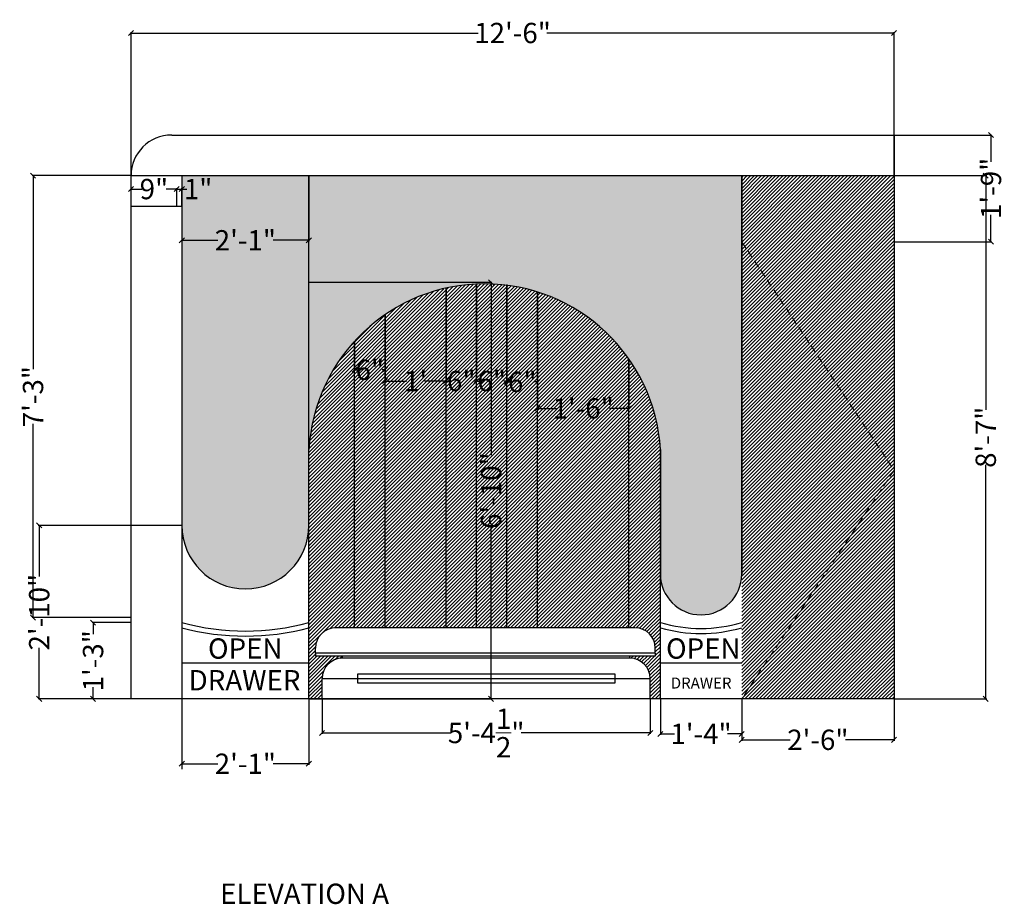
# Model space of a CAD drawing. Units: inches. Extents: x 1267 to 1461, y 390 to 564.
import ezdxf

# ---------------------------------------------------------------- set-up
doc = ezdxf.new("R2010")
doc.units = ezdxf.units.IN
doc.header["$LTSCALE"] = 3
doc.header["$MEASUREMENT"] = 0
doc.linetypes.add('DASHED', pattern=[0.75, 0.5, -0.25])
for name, color, linetype, lineweight in [('A-ANNO-DIMS', 2, 'Continuous', 18), ('A-ANNO-TEXT', 7, 'Continuous', 18), ('A-ELEV', 7, 'Continuous', 25), ('A-ELEV-HIDN', 8, 'DASHED', 18), ('A-ELEV-PATT', 8, 'Continuous', 13)]:
    doc.layers.add(name, color=color, linetype=linetype, lineweight=lineweight)
doc.styles.get("Standard").update_dxf_attribs({"font": 'arial.ttf'})
doc.dimstyles.get("Standard").update_dxf_attribs({"dimtxt": 4, "dimasz": 1, "dimexe": 0.18, "dimexo": 0.0625, "dimgap": 0.09, "dimtad": 0, "dimdec": 1, "dimzin": 0, "dimdsep": 46, "dimlunit": 4, "dimtxsty": 'Standard', "dimblk": 'OBLIQUE', "dimcen": 0.09, "dimadec": 0, "dimazin": 0, "dimtfac": 1, "dimtdec": 1, "dimtofl": 0, "dimtmove": 0, "dimatfit": 3, "dimldrblk": 'OBLIQUE', "dimfxl": 1, "dimtolj": 1, "dimtzin": 0, "dimarcsym": 0})

# ---------------------------------------------------------------- blocks, each defined once
blk = doc.blocks.new('_Oblique')
at = {"color": 0, "linetype": 'ByBlock', "lineweight": -2}
blk.add_line((-0.5, -0.5), (0.5, 0.5), dxfattribs=at)
blk = doc.blocks.new('*D2')
at = {"layer": 'A-ANNO-DIMS', "color": 0, "lineweight": -2, "transparency": 16777216}
for p, q in [((1439.3, 541.52), (1458.5, 541.52)), ((1458.32, 541.52), (1458.32, 536.24)), ((1458.32, 520.52), (1458.32, 525.8)), ((1439.3, 520.52), (1458.5, 520.52))]:
    blk.add_line(p, q, dxfattribs=at)
at = {"layer": 'Defpoints', "color": 0, "transparency": 16777216}
for p in [(1439.24, 541.52), (1439.24, 520.52), (1458.32, 520.52)]:
    blk.add_point(p, dxfattribs=at)
at = {"layer": 'A-ANNO-DIMS', "color": 0, "lineweight": -2, "transparency": 16777216}
for p, rotation in [((1458.32, 541.52), 90), ((1458.32, 520.52), 270)]:
    blk.add_blockref('_Oblique', p, dxfattribs=dict(at, rotation=rotation))
at = {"layer": 'A-ANNO-DIMS', "color": 0, "transparency": 16777216, "insert": (1458.32, 531.02), "char_height": 4, "attachment_point": 5, "rotation": 90}
blk.add_mtext('\\A1;1\'-9"', dxfattribs=at)
blk = doc.blocks.new('*D3')
at = {"layer": 'A-ANNO-DIMS', "color": 0, "lineweight": -2, "transparency": 16777216}
for p, q in [((1299.04, 430.46), (1299.04, 417.56)), ((1324.04, 430.46), (1324.04, 417.56)), ((1299.04, 417.74), (1306.1, 417.74)), ((1324.04, 417.74), (1316.98, 417.74))]:
    blk.add_line(p, q, dxfattribs=at)
at = {"layer": 'Defpoints', "color": 0, "transparency": 16777216}
for p in [(1299.04, 430.52), (1324.04, 430.52), (1299.04, 417.74)]:
    blk.add_point(p, dxfattribs=at)
at = {"layer": 'A-ANNO-DIMS', "color": 0, "lineweight": -2, "transparency": 16777216, "rotation": 180}
blk.add_blockref('_Oblique', (1299.04, 417.74), dxfattribs=at)
at = {"layer": 'A-ANNO-DIMS', "color": 0, "lineweight": -2, "transparency": 16777216}
blk.add_blockref('_Oblique', (1324.04, 417.74), dxfattribs=at)
at = {"layer": 'A-ANNO-DIMS', "color": 0, "transparency": 16777216, "insert": (1311.54, 417.74), "char_height": 4, "attachment_point": 5}
blk.add_mtext('\\A1;2\'-1"', dxfattribs=at)
blk = doc.blocks.new('*D4')
at = {"layer": 'A-ANNO-DIMS', "color": 0, "lineweight": -2, "transparency": 16777216}
for p, q in [((1326.64, 430.46), (1326.64, 423.62)), ((1391.24, 430.46), (1391.24, 423.62)), ((1326.64, 423.8), (1352.07, 423.8)), ((1391.24, 423.8), (1365.8, 423.8))]:
    blk.add_line(p, q, dxfattribs=at)
at = {"layer": 'Defpoints', "color": 0, "transparency": 16777216}
for p in [(1326.64, 430.52), (1391.24, 430.52), (1326.64, 423.8)]:
    blk.add_point(p, dxfattribs=at)
at = {"layer": 'A-ANNO-DIMS', "color": 0, "lineweight": -2, "transparency": 16777216, "rotation": 180}
blk.add_blockref('_Oblique', (1326.64, 423.8), dxfattribs=at)
at = {"layer": 'A-ANNO-DIMS', "color": 0, "lineweight": -2, "transparency": 16777216}
blk.add_blockref('_Oblique', (1391.24, 423.8), dxfattribs=at)
at = {"layer": 'A-ANNO-DIMS', "color": 0, "transparency": 16777216, "insert": (1358.94, 423.8), "char_height": 4, "attachment_point": 5}
blk.add_mtext('\\A1;5\'-4{\\H1x;\\S1/2;}"', dxfattribs=at)
blk = doc.blocks.new('*D5')
at = {"layer": 'A-ANNO-DIMS', "color": 0, "lineweight": -2, "transparency": 16777216}
for p, q in [((1393.24, 430.46), (1393.24, 423.44)), ((1409.24, 430.46), (1409.24, 423.44)), ((1393.24, 423.62), (1396.02, 423.62)), ((1409.24, 423.62), (1406.45, 423.62))]:
    blk.add_line(p, q, dxfattribs=at)
at = {"layer": 'Defpoints', "color": 0, "transparency": 16777216}
for p in [(1393.24, 430.52), (1409.24, 430.52), (1393.24, 423.62)]:
    blk.add_point(p, dxfattribs=at)
at = {"layer": 'A-ANNO-DIMS', "color": 0, "lineweight": -2, "transparency": 16777216, "rotation": 180}
blk.add_blockref('_Oblique', (1393.24, 423.62), dxfattribs=at)
at = {"layer": 'A-ANNO-DIMS', "color": 0, "lineweight": -2, "transparency": 16777216}
blk.add_blockref('_Oblique', (1409.24, 423.62), dxfattribs=at)
at = {"layer": 'A-ANNO-DIMS', "color": 0, "transparency": 16777216, "insert": (1401.24, 423.62), "char_height": 4, "attachment_point": 5}
blk.add_mtext('\\A1;1\'-4"', dxfattribs=at)
blk = doc.blocks.new('*D6')
at = {"layer": 'A-ANNO-DIMS', "color": 0, "lineweight": -2, "transparency": 16777216}
for p, q in [((1409.24, 430.46), (1409.24, 422.28)), ((1439.24, 430.46), (1439.24, 422.28)), ((1409.24, 422.46), (1418.8, 422.46)), ((1439.24, 422.46), (1429.68, 422.46))]:
    blk.add_line(p, q, dxfattribs=at)
at = {"layer": 'Defpoints', "color": 0, "transparency": 16777216}
for p in [(1409.24, 430.52), (1439.24, 430.52), (1409.24, 422.46)]:
    blk.add_point(p, dxfattribs=at)
at = {"layer": 'A-ANNO-DIMS', "color": 0, "lineweight": -2, "transparency": 16777216, "rotation": 180}
blk.add_blockref('_Oblique', (1409.24, 422.46), dxfattribs=at)
at = {"layer": 'A-ANNO-DIMS', "color": 0, "lineweight": -2, "transparency": 16777216}
blk.add_blockref('_Oblique', (1439.24, 422.46), dxfattribs=at)
at = {"layer": 'A-ANNO-DIMS', "color": 0, "transparency": 16777216, "insert": (1424.24, 422.46), "char_height": 4, "attachment_point": 5}
blk.add_mtext('\\A1;2\'-6"', dxfattribs=at)
blk = doc.blocks.new('*D7')
at = {"layer": 'A-ANNO-DIMS', "color": 0, "lineweight": -2, "transparency": 16777216}
for p, q in [((1289.04, 533.58), (1289.04, 561.78)), ((1289.04, 561.6), (1357.36, 561.6)), ((1439.24, 561.6), (1370.91, 561.6)), ((1439.24, 533.58), (1439.24, 561.78))]:
    blk.add_line(p, q, dxfattribs=at)
at = {"layer": 'Defpoints', "color": 0, "transparency": 16777216}
for p in [(1439.24, 561.6), (1289.04, 533.52), (1439.24, 533.52)]:
    blk.add_point(p, dxfattribs=at)
at = {"layer": 'A-ANNO-DIMS', "color": 0, "lineweight": -2, "transparency": 16777216, "rotation": 180}
blk.add_blockref('_Oblique', (1289.04, 561.6), dxfattribs=at)
at = {"layer": 'A-ANNO-DIMS', "color": 0, "lineweight": -2, "transparency": 16777216}
blk.add_blockref('_Oblique', (1439.24, 561.6), dxfattribs=at)
at = {"layer": 'A-ANNO-DIMS', "color": 0, "transparency": 16777216, "insert": (1364.14, 561.6), "char_height": 4, "attachment_point": 5}
blk.add_mtext('\\A1;12\'-6"', dxfattribs=at)
blk = doc.blocks.new('*D8')
at = {"layer": 'A-ANNO-DIMS', "color": 0, "lineweight": -2, "transparency": 16777216}
for p, q in [((1289.04, 527.58), (1289.04, 531.06)), ((1289.04, 530.88), (1291.15, 530.88)), ((1298.04, 530.88), (1295.93, 530.88)), ((1298.04, 527.58), (1298.04, 531.06))]:
    blk.add_line(p, q, dxfattribs=at)
at = {"layer": 'Defpoints', "color": 0, "transparency": 16777216}
for p in [(1298.04, 530.88), (1289.04, 527.52), (1298.04, 527.52)]:
    blk.add_point(p, dxfattribs=at)
at = {"layer": 'A-ANNO-DIMS', "color": 0, "lineweight": -2, "transparency": 16777216, "rotation": 180}
blk.add_blockref('_Oblique', (1289.04, 530.88), dxfattribs=at)
at = {"layer": 'A-ANNO-DIMS', "color": 0, "lineweight": -2, "transparency": 16777216}
blk.add_blockref('_Oblique', (1298.04, 530.88), dxfattribs=at)
at = {"layer": 'A-ANNO-DIMS', "color": 0, "transparency": 16777216, "insert": (1293.54, 530.88), "char_height": 4, "attachment_point": 5}
blk.add_mtext('\\A1;9"', dxfattribs=at)
blk = doc.blocks.new('*D9')
at = {"layer": 'A-ANNO-DIMS', "color": 0, "lineweight": -2, "transparency": 16777216}
for p, q in [((1298.04, 527.58), (1298.04, 531.06)), ((1298.04, 530.88), (1299.04, 530.88)), ((1299.04, 527.58), (1299.04, 531.06)), ((1299.04, 530.88), (1300.04, 530.88))]:
    blk.add_line(p, q, dxfattribs=at)
at = {"layer": 'Defpoints', "color": 0, "transparency": 16777216}
for p in [(1299.04, 530.88), (1298.04, 527.52), (1299.04, 527.52)]:
    blk.add_point(p, dxfattribs=at)
at = {"layer": 'A-ANNO-DIMS', "color": 0, "lineweight": -2, "transparency": 16777216, "rotation": 180}
blk.add_blockref('_Oblique', (1298.04, 530.88), dxfattribs=at)
at = {"layer": 'A-ANNO-DIMS', "color": 0, "lineweight": -2, "transparency": 16777216}
blk.add_blockref('_Oblique', (1299.04, 530.88), dxfattribs=at)
at = {"layer": 'A-ANNO-DIMS', "color": 0, "transparency": 16777216, "insert": (1302.24, 530.88), "char_height": 4, "attachment_point": 5}
blk.add_mtext('\\A1;1"', dxfattribs=at)
blk = doc.blocks.new('*D10')
at = {"layer": 'A-ANNO-DIMS', "color": 0, "lineweight": -2, "transparency": 16777216}
for p, q in [((1298.97, 464.66), (1270.77, 464.66)), ((1270.95, 464.66), (1270.95, 454.58)), ((1270.95, 430.52), (1270.95, 440.59)), ((1298.97, 430.52), (1270.77, 430.52))]:
    blk.add_line(p, q, dxfattribs=at)
at = {"layer": 'Defpoints', "color": 0, "transparency": 16777216}
for p in [(1299.04, 464.66), (1270.95, 430.52), (1299.04, 430.52)]:
    blk.add_point(p, dxfattribs=at)
at = {"layer": 'A-ANNO-DIMS', "color": 0, "lineweight": -2, "transparency": 16777216}
for p, rotation in [((1270.95, 464.66), 90), ((1270.95, 430.52), 270)]:
    blk.add_blockref('_Oblique', p, dxfattribs=dict(at, rotation=rotation))
at = {"layer": 'A-ANNO-DIMS', "color": 0, "transparency": 16777216, "insert": (1270.95, 447.59), "char_height": 4, "attachment_point": 5, "rotation": 90}
blk.add_mtext('\\A1;2\'-10"', dxfattribs=at)
blk = doc.blocks.new('*D11')
at = {"layer": 'A-ANNO-DIMS', "color": 0, "lineweight": -2, "transparency": 16777216}
for p, q in [((1288.97, 533.52), (1269.56, 533.52)), ((1269.74, 533.52), (1269.74, 495.41)), ((1269.74, 446.52), (1269.74, 484.63)), ((1288.97, 446.52), (1269.56, 446.52))]:
    blk.add_line(p, q, dxfattribs=at)
at = {"layer": 'Defpoints', "color": 0, "transparency": 16777216}
for p in [(1269.74, 533.52), (1289.04, 533.52), (1289.04, 446.52)]:
    blk.add_point(p, dxfattribs=at)
at = {"layer": 'A-ANNO-DIMS', "color": 0, "lineweight": -2, "transparency": 16777216}
for p, rotation in [((1269.74, 533.52), 90), ((1269.74, 446.52), 270)]:
    blk.add_blockref('_Oblique', p, dxfattribs=dict(at, rotation=rotation))
at = {"layer": 'A-ANNO-DIMS', "color": 0, "transparency": 16777216, "insert": (1269.74, 490.02), "char_height": 4, "attachment_point": 5, "rotation": 90}
blk.add_mtext('\\A1;7\'-3"', dxfattribs=at)
blk = doc.blocks.new('*D12')
at = {"layer": 'A-ANNO-DIMS', "color": 0, "lineweight": -2, "transparency": 16777216}
for p, q in [((1288.97, 445.52), (1281.38, 445.52)), ((1281.56, 445.52), (1281.56, 443.24)), ((1281.56, 430.52), (1281.56, 432.8)), ((1288.97, 430.52), (1281.38, 430.52))]:
    blk.add_line(p, q, dxfattribs=at)
at = {"layer": 'Defpoints', "color": 0, "transparency": 16777216}
for p in [(1281.56, 445.52), (1289.04, 445.52), (1289.04, 430.52)]:
    blk.add_point(p, dxfattribs=at)
at = {"layer": 'A-ANNO-DIMS', "color": 0, "lineweight": -2, "transparency": 16777216}
for p, rotation in [((1281.56, 445.52), 90), ((1281.56, 430.52), 270)]:
    blk.add_blockref('_Oblique', p, dxfattribs=dict(at, rotation=rotation))
at = {"layer": 'A-ANNO-DIMS', "color": 0, "transparency": 16777216, "insert": (1281.56, 438.02), "char_height": 4, "attachment_point": 5, "rotation": 90}
blk.add_mtext('\\A1;1\'-3"', dxfattribs=at)
blk = doc.blocks.new('*D13')
at = {"layer": 'A-ANNO-DIMS', "color": 0, "lineweight": -2, "transparency": 16777216}
for p, q in [((1339.04, 506.08), (1339.04, 495.13)), ((1333.04, 500.86), (1333.04, 495.13)), ((1333.04, 495.31), (1333.64, 495.31)), ((1339.04, 495.31), (1338.44, 495.31))]:
    blk.add_line(p, q, dxfattribs=at)
at = {"layer": 'Defpoints', "color": 0, "transparency": 16777216}
for p in [(1339.04, 506.14), (1333.04, 500.92), (1339.04, 495.31)]:
    blk.add_point(p, dxfattribs=at)
at = {"layer": 'A-ANNO-DIMS', "color": 0, "lineweight": -2, "transparency": 16777216, "rotation": 180}
blk.add_blockref('_Oblique', (1333.04, 495.31), dxfattribs=at)
at = {"layer": 'A-ANNO-DIMS', "color": 0, "lineweight": -2, "transparency": 16777216}
blk.add_blockref('_Oblique', (1339.04, 495.31), dxfattribs=at)
at = {"layer": 'A-ANNO-DIMS', "color": 0, "transparency": 16777216, "insert": (1336.04, 495.31), "char_height": 4, "attachment_point": 5}
blk.add_mtext('\\A1;6"', dxfattribs=at)
blk = doc.blocks.new('*D14')
at = {"layer": 'A-ANNO-DIMS', "color": 0, "lineweight": -2, "transparency": 16777216}
for p, q in [((1351.04, 511.31), (1351.04, 492.91)), ((1339.04, 495.24), (1339.04, 492.91)), ((1339.04, 493.09), (1343.29, 493.09)), ((1351.04, 493.09), (1346.78, 493.09))]:
    blk.add_line(p, q, dxfattribs=at)
at = {"layer": 'Defpoints', "color": 0, "transparency": 16777216}
for p in [(1351.04, 511.37), (1339.04, 495.31), (1351.04, 493.09)]:
    blk.add_point(p, dxfattribs=at)
at = {"layer": 'A-ANNO-DIMS', "color": 0, "lineweight": -2, "transparency": 16777216, "rotation": 180}
blk.add_blockref('_Oblique', (1339.04, 493.09), dxfattribs=at)
at = {"layer": 'A-ANNO-DIMS', "color": 0, "lineweight": -2, "transparency": 16777216}
blk.add_blockref('_Oblique', (1351.04, 493.09), dxfattribs=at)
at = {"layer": 'A-ANNO-DIMS', "color": 0, "transparency": 16777216, "insert": (1345.04, 493.09), "char_height": 4, "attachment_point": 5}
blk.add_mtext("\\A1;1'", dxfattribs=at)
blk = doc.blocks.new('*D15')
at = {"layer": 'A-ANNO-DIMS', "color": 0, "lineweight": -2, "transparency": 16777216}
for p, q in [((1357.04, 512.12), (1357.04, 492.91)), ((1351.04, 511.31), (1351.04, 492.91)), ((1351.04, 493.09), (1351.64, 493.09)), ((1357.04, 493.09), (1356.44, 493.09))]:
    blk.add_line(p, q, dxfattribs=at)
at = {"layer": 'Defpoints', "color": 0, "transparency": 16777216}
for p in [(1357.04, 512.18), (1351.04, 511.37), (1357.04, 493.09)]:
    blk.add_point(p, dxfattribs=at)
at = {"layer": 'A-ANNO-DIMS', "color": 0, "lineweight": -2, "transparency": 16777216, "rotation": 180}
blk.add_blockref('_Oblique', (1351.04, 493.09), dxfattribs=at)
at = {"layer": 'A-ANNO-DIMS', "color": 0, "lineweight": -2, "transparency": 16777216}
blk.add_blockref('_Oblique', (1357.04, 493.09), dxfattribs=at)
at = {"layer": 'A-ANNO-DIMS', "color": 0, "transparency": 16777216, "insert": (1354.04, 493.09), "char_height": 4, "attachment_point": 5}
blk.add_mtext('\\A1;6"', dxfattribs=at)
blk = doc.blocks.new('*D16')
at = {"layer": 'A-ANNO-DIMS', "color": 0, "lineweight": -2, "transparency": 16777216}
for p, q in [((1357.04, 512.12), (1357.04, 492.91)), ((1363.04, 512.12), (1363.04, 492.91)), ((1357.04, 493.09), (1357.64, 493.09)), ((1363.04, 493.09), (1362.44, 493.09))]:
    blk.add_line(p, q, dxfattribs=at)
at = {"layer": 'Defpoints', "color": 0, "transparency": 16777216}
for p in [(1357.04, 512.18), (1363.04, 512.18), (1363.04, 493.09)]:
    blk.add_point(p, dxfattribs=at)
at = {"layer": 'A-ANNO-DIMS', "color": 0, "lineweight": -2, "transparency": 16777216, "rotation": 180}
blk.add_blockref('_Oblique', (1357.04, 493.09), dxfattribs=at)
at = {"layer": 'A-ANNO-DIMS', "color": 0, "lineweight": -2, "transparency": 16777216}
blk.add_blockref('_Oblique', (1363.04, 493.09), dxfattribs=at)
at = {"layer": 'A-ANNO-DIMS', "color": 0, "transparency": 16777216, "insert": (1360.04, 493.09), "char_height": 4, "attachment_point": 5}
blk.add_mtext('\\A1;6"', dxfattribs=at)
blk = doc.blocks.new('*D17')
at = {"layer": 'A-ANNO-DIMS', "color": 0, "lineweight": -2, "transparency": 16777216}
for p, q in [((1363.04, 511.87), (1363.04, 492.73)), ((1369.04, 510.56), (1369.04, 492.73)), ((1363.04, 492.91), (1363.64, 492.91)), ((1369.04, 492.91), (1368.44, 492.91))]:
    blk.add_line(p, q, dxfattribs=at)
at = {"layer": 'Defpoints', "color": 0, "transparency": 16777216}
for p in [(1363.04, 511.94), (1369.04, 510.62), (1369.04, 492.91)]:
    blk.add_point(p, dxfattribs=at)
at = {"layer": 'A-ANNO-DIMS', "color": 0, "lineweight": -2, "transparency": 16777216, "rotation": 180}
blk.add_blockref('_Oblique', (1363.04, 492.91), dxfattribs=at)
at = {"layer": 'A-ANNO-DIMS', "color": 0, "lineweight": -2, "transparency": 16777216}
blk.add_blockref('_Oblique', (1369.04, 492.91), dxfattribs=at)
at = {"layer": 'A-ANNO-DIMS', "color": 0, "transparency": 16777216, "insert": (1366.04, 492.91), "char_height": 4, "attachment_point": 5}
blk.add_mtext('\\A1;6"', dxfattribs=at)
blk = doc.blocks.new('*D18')
at = {"layer": 'A-ANNO-DIMS', "color": 0, "lineweight": -2, "transparency": 16777216}
for p, q in [((1369.04, 510.56), (1369.04, 487.53)), ((1387.04, 497.36), (1387.04, 487.53)), ((1369.04, 487.71), (1372.82, 487.71)), ((1387.04, 487.71), (1383.25, 487.71))]:
    blk.add_line(p, q, dxfattribs=at)
at = {"layer": 'Defpoints', "color": 0, "transparency": 16777216}
for p in [(1369.04, 510.62), (1387.04, 497.42), (1387.04, 487.71)]:
    blk.add_point(p, dxfattribs=at)
at = {"layer": 'A-ANNO-DIMS', "color": 0, "lineweight": -2, "transparency": 16777216, "rotation": 180}
blk.add_blockref('_Oblique', (1369.04, 487.71), dxfattribs=at)
at = {"layer": 'A-ANNO-DIMS', "color": 0, "lineweight": -2, "transparency": 16777216}
blk.add_blockref('_Oblique', (1387.04, 487.71), dxfattribs=at)
at = {"layer": 'A-ANNO-DIMS', "color": 0, "transparency": 16777216, "insert": (1378.04, 487.71), "char_height": 4, "attachment_point": 5}
blk.add_mtext('\\A1;1\'-6"', dxfattribs=at)
blk = doc.blocks.new('*D19')
at = {"layer": 'A-ANNO-DIMS', "color": 0, "lineweight": -2, "transparency": 16777216}
for p, q in [((1299.04, 533.46), (1299.04, 520.61)), ((1324.04, 533.46), (1324.04, 520.61)), ((1299.04, 520.79), (1306.1, 520.79)), ((1324.04, 520.79), (1316.98, 520.79))]:
    blk.add_line(p, q, dxfattribs=at)
at = {"layer": 'Defpoints', "color": 0, "transparency": 16777216}
for p in [(1299.04, 533.52), (1324.04, 533.52), (1324.04, 520.79)]:
    blk.add_point(p, dxfattribs=at)
at = {"layer": 'A-ANNO-DIMS', "color": 0, "lineweight": -2, "transparency": 16777216, "rotation": 180}
blk.add_blockref('_Oblique', (1299.04, 520.79), dxfattribs=at)
at = {"layer": 'A-ANNO-DIMS', "color": 0, "lineweight": -2, "transparency": 16777216}
blk.add_blockref('_Oblique', (1324.04, 520.79), dxfattribs=at)
at = {"layer": 'A-ANNO-DIMS', "color": 0, "transparency": 16777216, "insert": (1311.54, 520.79), "char_height": 4, "attachment_point": 5}
blk.add_mtext('\\A1;2\'-1"', dxfattribs=at)
blk = doc.blocks.new('*D20')
at = {"layer": 'A-ANNO-DIMS', "color": 0, "lineweight": -2, "transparency": 16777216}
for p, q in [((1324.1, 512.52), (1360.09, 512.52)), ((1359.91, 512.52), (1359.91, 478.49)), ((1359.91, 430.52), (1359.91, 464.55)), ((1324.1, 430.52), (1360.09, 430.52))]:
    blk.add_line(p, q, dxfattribs=at)
at = {"layer": 'Defpoints', "color": 0, "transparency": 16777216}
for p in [(1324.04, 512.52), (1359.91, 512.52), (1324.04, 430.52)]:
    blk.add_point(p, dxfattribs=at)
at = {"layer": 'A-ANNO-DIMS', "color": 0, "lineweight": -2, "transparency": 16777216}
for p, rotation in [((1359.91, 512.52), 90), ((1359.91, 430.52), 270)]:
    blk.add_blockref('_Oblique', p, dxfattribs=dict(at, rotation=rotation))
at = {"layer": 'A-ANNO-DIMS', "color": 0, "transparency": 16777216, "insert": (1359.91, 471.52), "char_height": 4, "attachment_point": 5, "rotation": 90}
blk.add_mtext('\\A1;6\'-10"', dxfattribs=at)
blk = doc.blocks.new('*D21')
at = {"layer": 'A-ANNO-DIMS', "color": 0, "lineweight": -2, "transparency": 16777216}
for p, q in [((1439.3, 533.52), (1457.47, 533.52)), ((1457.29, 533.52), (1457.29, 487.43)), ((1457.29, 430.52), (1457.29, 476.61)), ((1439.3, 430.52), (1457.47, 430.52))]:
    blk.add_line(p, q, dxfattribs=at)
at = {"layer": 'Defpoints', "color": 0, "transparency": 16777216}
for p in [(1439.24, 533.52), (1439.24, 430.52), (1457.29, 430.52)]:
    blk.add_point(p, dxfattribs=at)
at = {"layer": 'A-ANNO-DIMS', "color": 0, "lineweight": -2, "transparency": 16777216}
for p, rotation in [((1457.29, 533.52), 90), ((1457.29, 430.52), 270)]:
    blk.add_blockref('_Oblique', p, dxfattribs=dict(at, rotation=rotation))
at = {"layer": 'A-ANNO-DIMS', "color": 0, "transparency": 16777216, "insert": (1457.29, 482.02), "char_height": 4, "attachment_point": 5, "rotation": 90}
blk.add_mtext('\\A1;8\'-7"', dxfattribs=at)

msp = doc.modelspace()

# ---------------------------------------------------------------- hatches: boundary and pattern name
at = {"layer": 'A-ELEV-PATT'}
h = msp.add_hatch(color=256, dxfattribs=at)
h.dxf.hatch_style = 1
h.set_gradient(color1=(255, 255, 255), color2=(0, 127, 255), name='CYLINDER')
h.paths.add_polyline_path([(1324.04, 533.52), (1299.04, 533.52), (1299.04, 464.66, 1), (1324.04, 464.66)])
h.paths.add_polyline_path([(1298.52, 526.7), (1305.61, 526.7), (1305.61, 534.94), (1298.52, 534.94)], flags=9)
h.paths.add_polyline_path([(1305.02, 516.6), (1318.15, 516.6), (1318.15, 524.85), (1305.02, 524.85)], flags=24)
h = msp.add_hatch(color=256, dxfattribs=at)
h.dxf.hatch_style = 1
h.paths.add_polyline_path([(1393.24, 479.59), (1393.24, 455.06, 1), (1409.24, 455.06), (1409.24, 533.52), (1324.04, 533.52), (1324.04, 479.59, -0.942896)])
h = msp.add_hatch(dxfattribs=at)
h.set_pattern_fill('ANSI31', color=256, scale=4)
h.paths.add_polyline_path([(1439.24, 520.52), (1439.24, 533.52), (1409.24, 533.52), (1409.24, 520.52), (1439.24, 475.52)])
h.paths.add_polyline_path([(1409.24, 520.52), (1409.24, 430.52), (1439.24, 475.52)])
h.paths.add_polyline_path([(1439.24, 475.52), (1409.24, 430.52), (1439.24, 430.52)], flags=17)
h.paths.add_polyline_path([(1392.86, 436.17), (1410.7, 436.17), (1410.7, 444.42), (1392.86, 444.42)], flags=9)
h = msp.add_hatch(dxfattribs=at)
h.set_pattern_fill('ANSI31', color=256, scale=4)
h.paths.add_polyline_path([(1333.04, 500.92, 0.171922), (1324.04, 479.59), (1324.04, 430.52), (1326.64, 430.52), (1326.64, 434.52, -0.414214), (1330.64, 438.52), (1330.64, 438.92), (1325.34, 438.92), (1325.34, 439.52), (1325.34, 440.52, -0.414214), (1329.34, 444.52), (1333.04, 444.52)])
h.paths.add_polyline_path([(1339.04, 506.14, 0.057555), (1333.04, 500.92), (1333.04, 444.52), (1339.04, 444.52)])
h.paths.add_polyline_path([(1351.04, 511.37, 0.095278), (1339.04, 506.14), (1339.04, 444.52), (1351.04, 444.52)])
h.paths.add_polyline_path([(1357.04, 512.18, 0.043751), (1351.04, 511.37), (1351.04, 444.52), (1357.04, 444.52)])
h.paths.add_polyline_path([(1363.04, 511.94, 0.043395), (1357.04, 512.18), (1357.04, 444.52), (1363.04, 444.52)])
h.paths.add_polyline_path([(1369.04, 510.62, 0.044395), (1363.04, 511.94), (1363.04, 444.52), (1369.04, 444.52)])
h.paths.add_polyline_path([(1387.04, 497.42, 0.165382), (1369.04, 510.62), (1369.04, 444.52), (1387.04, 444.52)])
h.paths.add_polyline_path([(1393.24, 479.59, 0.138801), (1387.04, 497.42), (1387.04, 444.52), (1388.24, 444.52, -0.414214), (1392.24, 440.52), (1392.24, 439.52), (1392.24, 438.92), (1387.24, 438.92), (1387.24, 438.52, -0.414214), (1391.24, 434.52), (1391.24, 430.52), (1393.24, 430.52)])

# ---------------------------------------------------------------- linework, layer by layer
at = {"layer": 'A-ELEV'}
for p, q in [((1297.04, 541.52), (1325.64, 541.52)), ((1325.64, 541.52), (1409.24, 541.52)), ((1409.24, 541.52), (1439.24, 541.52)), ((1439.24, 541.52), (1439.24, 520.52)), ((1289.04, 446.52), (1289.04, 533.52)), ((1289.04, 527.52), (1289.04, 533.52)), ((1289.04, 533.52), (1439.24, 533.52)), ((1299.04, 533.52), (1299.04, 464.66)), ((1324.04, 464.66), (1324.04, 533.52)), ((1409.24, 533.52), (1409.24, 455.06)), ((1409.24, 455.06), (1409.24, 533.52)), ((1289.04, 527.52), (1298.04, 527.52)), ((1298.04, 527.52), (1299.04, 527.52)), ((1439.24, 520.52), (1439.24, 430.52)), ((1357.04, 444.52), (1357.04, 512.18)), ((1363.04, 444.52), (1363.04, 511.94)), ((1351.04, 444.52), (1351.04, 511.37)), ((1369.04, 444.52), (1369.04, 510.62)), ((1339.04, 444.52), (1339.04, 506.14)), ((1333.04, 444.52), (1333.04, 500.92)), ((1387.04, 444.52), (1387.04, 497.42)), ((1324.04, 430.52), (1324.04, 479.59)), ((1393.24, 430.52), (1393.24, 479.59)), ((1393.24, 479.59), (1393.24, 455.06)), ((1299.04, 464.66), (1299.04, 430.52)), ((1289.04, 445.52), (1289.04, 446.52)), ((1299.04, 446.52), (1299.04, 416.67)), ((1289.04, 430.52), (1289.04, 445.52)), ((1388.24, 444.52), (1329.34, 444.52)), ((1325.34, 439.52), (1325.34, 440.52)), ((1392.24, 439.52), (1392.24, 440.52)), ((1392.24, 439.52), (1325.34, 439.52)), ((1325.34, 439.52), (1325.34, 438.92)), ((1392.24, 438.92), (1325.34, 438.92)), ((1330.64, 438.52), (1330.64, 438.92)), ((1387.24, 438.52), (1330.64, 438.52)), ((1387.24, 438.52), (1387.24, 438.92)), ((1392.24, 439.52), (1392.24, 438.92)), ((1324.04, 437.52), (1299.04, 437.52)), ((1409.24, 437.52), (1393.24, 437.52)), ((1326.64, 430.52), (1326.64, 434.52)), ((1326.64, 434.52), (1391.24, 434.52)), ((1391.24, 430.52), (1391.24, 434.52)), ((1298.04, 430.52), (1289.04, 430.52)), ((1299.04, 430.52), (1298.04, 430.52)), ((1324.04, 430.52), (1299.04, 430.52)), ((1326.64, 430.52), (1324.04, 430.52)), ((1391.24, 430.52), (1326.64, 430.52)), ((1393.24, 430.52), (1391.24, 430.52)), ((1409.24, 430.52), (1393.24, 430.52)), ((1439.24, 430.52), (1409.24, 430.52))]:
    msp.add_line(p, q, dxfattribs=at)
msp.add_lwpolyline([(1333.69, 435.45), (1384.3, 435.45), (1384.3, 433.61), (1333.69, 433.61)], close=True, dxfattribs=at)
for centre, radius, start, end in [((1297.04, 533.52), 8, 90, 180), ((1358.64, 477.56), 34.66, 3.367, 176.633), ((1311.54, 464.66), 12.5, 180, 0), ((1401.24, 455.06), 8, 180, 0), ((1311.54, 490.86), 46.99, 254.5737, 285.4263), ((1311.54, 490.86), 47.99, 254.9029, 285.0971), ((1329.34, 440.52), 4, 90, 180), ((1388.24, 440.52), 4, 0, 90), ((1401.24, 472.09), 27.71, 253.2185, 286.7815), ((1401.24, 472.09), 28.71, 253.8195, 286.1805), ((1330.64, 434.52), 4, 90, 180), ((1387.24, 434.52), 4, 0, 90)]:
    msp.add_arc(centre, radius, start, end, dxfattribs=at)
at = {"layer": 'A-ELEV-HIDN'}
for p, q in [((1409.24, 520.52), (1439.24, 475.52)), ((1439.24, 475.52), (1409.24, 430.52))]:
    msp.add_line(p, q, dxfattribs=at)

# ---------------------------------------------------------------- texts
at = {"layer": 'A-ANNO-TEXT', "attachment_point": 1}
for s, width, gutter_width, insert, char_height in [('\\pxqc;OPEN', 21.5955, 20, (1300.72, 442.43), 4), ('\\pxqc;OPEN', 21.5955, 20, (1390.89, 442.43), 4), ('\\pxqc;DRAWER', 22.9138, 20, (1299.92, 436.19), 4), ('\\pxqc;DRAWER', 12.4403, 10.86, (1395.04, 434.72), 2.1717), ('ELEVATION A', 121.8854, 20, (1306.57, 394.15), 4)]:
    msp.add_mtext_dynamic_manual_height_columns(s, width=width, gutter_width=gutter_width, heights=[0], dxfattribs=dict(at, insert=insert, char_height=char_height))

# ---------------------------------------------------------------- dimensions: what is measured, and where the dimension line sits
at = {"layer": 'A-ANNO-DIMS'}
for base, p1, p2, picture, middle in [((1439.24, 561.6), (1289.04, 533.52), (1439.24, 533.52), '*D7', (1364.14, 561.6)), ((1298.04, 530.88), (1289.04, 527.52), (1298.04, 527.52), '*D8', (1293.54, 530.88)), ((1299.04, 530.88), (1298.04, 527.52), (1299.04, 527.52), '*D9', (1302.24, 530.88)), ((1324.04, 520.79), (1299.04, 533.52), (1324.04, 533.52), '*D19', (1311.54, 520.79)), ((1357.04, 493.09), (1351.04, 511.37), (1357.04, 512.18), '*D15', (1354.04, 493.09)), ((1363.04, 493.09), (1357.04, 512.18), (1363.04, 512.18), '*D16', (1360.04, 493.09)), ((1369.04, 492.91), (1363.04, 511.94), (1369.04, 510.62), '*D17', (1366.04, 492.91)), ((1351.04, 493.09), (1339.04, 495.31), (1351.04, 511.37), '*D14', (1345.04, 493.09)), ((1387.04, 487.71), (1369.04, 510.62), (1387.04, 497.42), '*D18', (1378.04, 487.71)), ((1339.04, 495.31), (1333.04, 500.92), (1339.04, 506.14), '*D13', (1336.04, 495.31)), ((1299.04, 417.74), (1324.04, 430.52), (1299.04, 430.52), '*D3', (1311.54, 417.74)), ((1326.64, 423.8), (1391.24, 430.52), (1326.64, 430.52), '*D4', (1358.94, 423.8)), ((1393.24, 423.62), (1409.24, 430.52), (1393.24, 430.52), '*D5', (1401.24, 423.62)), ((1409.24, 422.46), (1439.24, 430.52), (1409.24, 430.52), '*D6', (1424.24, 422.46))]:
    dim = msp.add_linear_dim(base=base, p1=p1, p2=p2, dimstyle='Standard', override={"dimclrd": 0, "dimclre": 0, "dimclrt": 0}, dxfattribs=at)
    dim.commit()
    dim.dimension.update_dxf_attribs({"geometry": picture, "text_midpoint": middle})
for base, p1, p2, picture, middle in [((1458.32, 520.52), (1439.24, 541.52), (1439.24, 520.52), '*D2', (1458.32, 531.02)), ((1269.74, 533.52), (1289.04, 446.52), (1289.04, 533.52), '*D11', (1269.74, 490.02)), ((1457.29, 430.52), (1439.24, 533.52), (1439.24, 430.52), '*D21', (1457.29, 482.02)), ((1359.91, 512.52), (1324.04, 430.52), (1324.04, 512.52), '*D20', (1359.91, 471.52)), ((1270.95, 430.52), (1299.04, 464.66), (1299.04, 430.52), '*D10', (1270.95, 447.59)), ((1281.56, 445.52), (1289.04, 430.52), (1289.04, 445.52), '*D12', (1281.56, 438.02))]:
    dim = msp.add_linear_dim(base=base, p1=p1, p2=p2, angle=90, dimstyle='Standard', override={"dimclrd": 0, "dimclre": 0, "dimclrt": 0}, dxfattribs=at)
    dim.commit()
    dim.dimension.update_dxf_attribs({"geometry": picture, "text_midpoint": middle})

doc.saveas('drawing.dxf')
